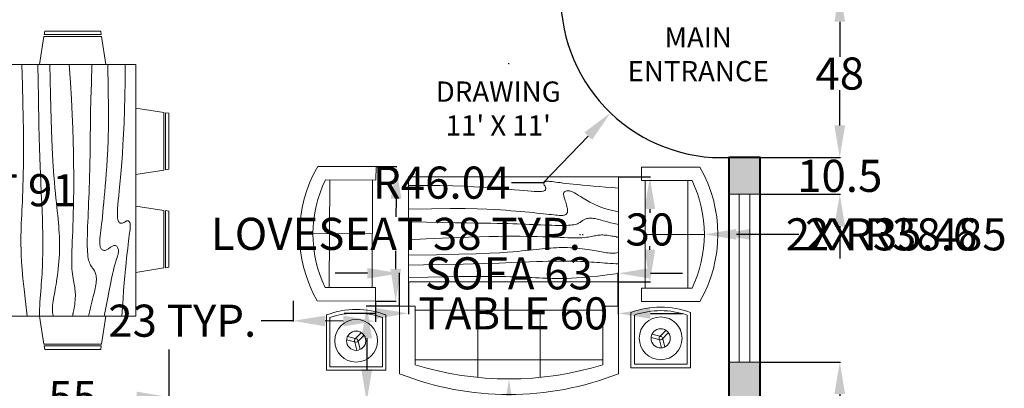
# Model space of a CAD drawing. Units: inches. Extents: x -51 to 563, y -59 to 453.
# Tile 5 of 6: x 211 to 492, y 134 to 240. Entities that reach past the tile are written whole.
import ezdxf

# ---------------------------------------------------------------- set-up
doc = ezdxf.new("R2010")
doc.units = ezdxf.units.IN
doc.header["$MEASUREMENT"] = 0
for name, color, linetype, lineweight in [('A-ANNO-DIMS', 2, 'Continuous', 18), ('A-AREA-IDEN', 7, 'Continuous', 25), ('A-DOOR', 3, 'Continuous', 25), ('A-FURN', 8, 'Continuous', 18), ('A-GLAZ', 4, 'Continuous', 18), ('A-WALL', 7, 'Continuous', 40), ('A-WALL-PATT', 252, 'Continuous', 13)]:
    doc.layers.add(name, color=color, linetype=linetype, lineweight=lineweight)
doc.styles.get("Standard").update_dxf_attribs({"font": 'arial.ttf'})
doc.dimstyles.get("Standard").update_dxf_attribs({"dimtxt": 9.18, "dimasz": 9.18, "dimexe": 0.18, "dimexo": 0.0625, "dimgap": 0.09, "dimtad": 0, "dimtih": 1, "dimtoh": 1, "dimdec": 1, "dimzin": 0, "dimdsep": 46, "dimlunit": 3, "dimtxsty": 'Standard', "dimcen": 0.09, "dimadec": 0, "dimazin": 0, "dimtfac": 1, "dimtdec": 1, "dimtofl": 0, "dimtmove": 0, "dimatfit": 3, "dimfxl": 1, "dimtolj": 1, "dimtzin": 0, "dimarcsym": 0})

# ---------------------------------------------------------------- blocks, each defined once
blk = doc.blocks.new('Dining Set - 36 x 72 in.')
for p, q in [((-22.2343, 26.00059), (-23.4847, 17.99762)), ((-22.2304, 26), (-5.7608, 26)), ((-22, 27.5), (-22.1562, 26.50042)), ((-5.8416, 26.5), (-22.1534, 26.5)), ((-22, 27.5), (-6, 27.5)), ((-5.8437, 26.49966), (-6, 27.5)), ((-4.5152, 17.99762), (-5.7655, 25.99926)), ((5.7657, 26.00059), (4.5153, 17.99762)), ((5.7696, 26), (22.2392, 26)), ((6, 27.5), (5.8438, 26.50042)), ((22.1584, 26.5), (5.8466, 26.5)), ((6, 27.5), (22, 27.5)), ((22.1563, 26.49966), (22, 27.5)), ((23.4848, 17.99762), (22.2345, 25.99926)), ((36, 18), (-36, 18)), ((-36, 18), (-36, -18)), ((36, -18), (36, 18)), ((-44.0006, 8.23428), (-35.9976, 9.48474)), ((44.0006, 8.23428), (35.9976, 9.48474)), ((-45.5, 8), (-44.5004, 8.15617)), ((-45.5, 8), (-45.5, -8)), ((-44.5, -8.15843), (-44.5, 8.15338)), ((-44, 8.23041), (-44, -8.23915)), ((44, 8.23041), (44, -8.23915)), ((44.5, -8.15843), (44.5, 8.15338)), ((45.5, 8), (44.5005, 8.15617)), ((45.5, 8), (45.5, -8)), ((-44.4997, -8.15631), (-45.5, -8)), ((-35.9976, -9.48476), (-43.9993, -8.2345)), ((35.9976, -9.48476), (43.9993, -8.2345)), ((44.4997, -8.15631), (45.5, -8)), ((-36, -18), (36, -18)), ((-22.2343, -26.0006), (-23.4847, -17.99762)), ((-4.5152, -17.99762), (-5.7655, -25.99928)), ((5.7657, -26.0006), (4.5153, -17.99762)), ((23.4848, -17.99762), (22.2345, -25.99928)), ((-22.2304, -26), (-5.7608, -26)), ((-22, -27.5), (-22.1562, -26.50044)), ((-5.8416, -26.5), (-22.1534, -26.5)), ((-22, -27.5), (-6, -27.5)), ((-5.8437, -26.49967), (-6, -27.5)), ((5.7696, -26), (22.2392, -26)), ((6, -27.5), (5.8438, -26.50044)), ((22.1584, -26.5), (5.8466, -26.5)), ((6, -27.5), (22, -27.5)), ((22.1563, -26.49967), (22, -27.5))]:
    blk.add_line(p, q)
for points in [[(-36, 15), (-31.1772, 14.97754), (-26.8079, 14.91406), (-22.8538, 14.81543), (-19.276, 14.6875), (-16.0362, 14.53613), (-13.0957, 14.36718), (-10.4159, 14.18652), (-7.9583, 14), (-5.6904, 13.81315), (-3.6035, 13.63021), (-1.6954, 13.45508), (0.0365, 13.29166), (1.5945, 13.14388), (2.9811, 13.01562), (4.1988, 12.9108), (5.25, 12.83333), (6.1393, 12.78613), (6.8802, 12.76823), (7.4883, 12.77767), (7.9792, 12.8125), (8.3685, 12.87077), (8.6719, 12.95052), (8.9049, 13.0498), (9.0833, 13.16666), (9.2205, 13.29899), (9.3216, 13.44401), (9.3895, 13.59879), (9.4271, 13.76041), (9.4373, 13.92594), (9.4232, 14.09245), (9.3875, 14.257), (9.3333, 14.41666), (9.2638, 14.56917), (9.1836, 14.71484), (9.0975, 14.85465), (9.0104, 14.98958), (8.9272, 15.1206), (8.8529, 15.2487), (8.7922, 15.37483), (8.75, 15.5), (8.7305, 15.62467), (8.7344, 15.74739), (8.7617, 15.86621), (8.8125, 15.97916), (8.8867, 16.08431), (8.9844, 16.17968), (9.1055, 16.26334), (9.25, 16.33333), (9.4189, 16.38802), (9.6172, 16.42708), (9.8506, 16.45052), (10.125, 16.45833), (10.4463, 16.45052), (10.8203, 16.42708), (11.2529, 16.38802), (11.75, 16.33333), (12.3184, 16.26318), (12.9694, 16.17838), (13.7151, 16.07991), (14.5677, 15.96875), (15.5395, 15.84586), (16.6426, 15.71224), (17.8893, 15.56884), (19.2917, 15.41666), (20.859, 15.25667), (22.5879, 15.08984), (24.4721, 14.91715), (26.5052, 14.73958), (28.6809, 14.5581), (30.9929, 14.3737), (33.4347, 14.18733), (36, 14)], [(-36, 10), (-28.9766, 10.14274), (-23.1725, 10.20442), (-18.4241, 10.19775), (-14.5677, 10.13541), (-11.4399, 10.03011), (-8.877, 9.89453), (-6.7154, 9.74137), (-4.7917, 9.58333), (-2.9698, 9.43082), (-1.2246, 9.28515), (0.4415, 9.14534), (2.026, 9.01041), (3.5266, 8.87939), (4.9408, 8.7513), (6.266, 8.62516), (7.5, 8.5), (8.6411, 8.37549), (9.6914, 8.2539), (10.6538, 8.13818), (11.5312, 8.03125), (12.3267, 7.93603), (13.043, 7.85547), (13.6831, 7.79248), (14.25, 7.75), (14.7471, 7.7303), (15.1797, 7.73307), (15.5537, 7.75732), (15.875, 7.80208), (16.1494, 7.86637), (16.3828, 7.94922), (16.5811, 8.04964), (16.75, 8.16666), (16.8944, 8.29915), (17.0143, 8.44531), (17.1089, 8.60319), (17.1771, 8.77083), (17.218, 8.94629), (17.2305, 9.1276), (17.2137, 9.31282), (17.1667, 9.5), (17.0895, 9.6875), (16.987, 9.875), (16.8649, 10.0625), (16.7292, 10.25), (16.5856, 10.4375), (16.4401, 10.625), (16.2985, 10.8125), (16.1667, 11), (16.05, 11.18733), (15.9518, 11.3737), (15.8752, 11.5581), (15.8229, 11.73958), (15.798, 11.91715), (15.8034, 12.08984), (15.842, 12.25667), (15.9167, 12.41666), (16.0295, 12.56836), (16.1784, 12.70833), (16.3605, 12.83268), (16.5729, 12.9375), (16.8127, 13.01888), (17.0768, 13.07291), (17.3625, 13.0957), (17.6667, 13.08333), (17.9894, 13.03312), (18.3418, 12.94726), (18.7382, 12.82918), (19.1927, 12.68229), (19.7195, 12.51001), (20.3327, 12.31575), (21.0465, 12.10294), (21.875, 11.875), (22.8357, 11.63354), (23.959, 11.37304), (25.2786, 11.08618), (26.8282, 10.76562), (28.6414, 10.40405), (30.752, 9.99414), (33.1936, 9.52856), (36, 9)], [(-36, 5.5), (-30.7157, 5.3348), (-26.069, 5.20963), (-21.9946, 5.11767), (-18.4271, 5.05208), (-15.3009, 5.00602), (-12.5508, 4.97265), (-10.1112, 4.94515), (-7.9167, 4.91666), (-5.909, 4.88167), (-4.0586, 4.83984), (-2.3429, 4.79215), (-0.7396, 4.73958), (0.7739, 4.6831), (2.22, 4.6237), (3.6213, 4.56233), (5, 4.5), (6.373, 4.43782), (7.7344, 4.3776), (9.0723, 4.32129), (10.375, 4.27083), (11.6309, 4.22819), (12.8281, 4.19531), (13.9551, 4.17415), (15, 4.16666), (15.954, 4.17448), (16.819, 4.19791), (17.6001, 4.23698), (18.3021, 4.29166), (18.9299, 4.36198), (19.4883, 4.44791), (19.9823, 4.54948), (20.4167, 4.66666), (20.7969, 4.79899), (21.1302, 4.94401), (21.4245, 5.09879), (21.6875, 5.26041), (21.9271, 5.42594), (22.1511, 5.59245), (22.3672, 5.757), (22.5834, 5.91666), (22.8065, 6.06868), (23.0404, 6.21093), (23.2879, 6.34147), (23.5521, 6.45833), (23.8358, 6.55957), (24.142, 6.64323), (24.4735, 6.70735), (24.8334, 6.75), (25.2235, 6.76969), (25.642, 6.76692), (26.0858, 6.74267), (26.5521, 6.69791), (27.0379, 6.63362), (27.5404, 6.55078), (28.0565, 6.45036), (28.5834, 6.33333), (29.1242, 6.19987), (29.7071, 6.04687), (30.3661, 5.87044), (31.1354, 5.66666), (32.0493, 5.43164), (33.142, 5.16146), (34.4475, 4.85221), (36, 4.5)], [(-36, -1), (-30.7915, -0.6591), (-26.0195, -0.38216), (-21.6519, -0.16284), (-17.6563, 0.00521), (-14.0005, 0.12833), (-10.6523, 0.21289), (-7.5796, 0.26522), (-4.75, 0.29166), (-2.134, 0.29793), (0.2878, 0.28711), (2.5317, 0.26163), (4.6146, 0.22396), (6.5529, 0.17651), (8.3633, 0.12174), (10.0623, 0.06209), (11.6667, 0), (13.1899, -0.06201), (14.6341, -0.1211), (15.9982, -0.17432), (17.2813, -0.21875), (18.4823, -0.25147), (19.6003, -0.26953), (20.6343, -0.27002), (21.5834, -0.25), (22.4481, -0.20768), (23.2357, -0.14584), (23.9549, -0.06836), (24.6146, 0.02083), (25.2235, 0.11784), (25.7904, 0.21875), (26.3241, 0.31966), (26.8334, 0.41666), (27.3265, 0.50618), (27.8099, 0.58593), (28.2894, 0.65397), (28.7709, 0.70833), (29.2601, 0.74707), (29.763, 0.76823), (30.2855, 0.76985), (30.8334, 0.75), (31.4088, 0.70784), (31.9994, 0.64713), (32.589, 0.57275), (33.1615, 0.48958), (33.7008, 0.4025), (34.1908, 0.3164), (34.6153, 0.23616), (34.9584, 0.16666), (35.2099, 0.11165), (35.3848, 0.07031), (35.504, 0.04069), (35.5886, 0.02083), (35.6594, 0.00879), (35.7377, 0.0026), (35.8442, 0.00032), (36, 0)], [(-36, -6.5), (-27.1843, -6.31267), (-20.084, -6.1263), (-14.469, -5.9419), (-10.1094, -5.76042), (-6.7752, -5.58285), (-4.2363, -5.41016), (-2.2629, -5.24333), (-0.625, -5.08334), (0.8708, -4.93099), (2.2715, -4.78646), (3.5872, -4.64974), (4.8281, -4.52084), (6.0046, -4.39974), (7.127, -4.28646), (8.2053, -4.18099), (9.25, -4.08334), (10.2705, -3.99382), (11.2734, -3.91407), (12.2647, -3.84603), (13.25, -3.79167), (14.2354, -3.75293), (15.2266, -3.73177), (16.2295, -3.73015), (17.25, -3.75), (18.2912, -3.79248), (19.3451, -3.85547), (20.4009, -3.93604), (21.4479, -4.03125), (22.4754, -4.13819), (23.4727, -4.25391), (24.4289, -4.37549), (25.3334, -4.5), (26.1785, -4.62492), (26.9694, -4.74935), (27.7145, -4.87281), (28.4219, -4.99479), (29.1, -5.11483), (29.7572, -5.23242), (30.4016, -5.34709), (31.0417, -5.45834), (31.6837, -5.56437), (32.3262, -5.65821), (32.9658, -5.73153), (33.599, -5.77604), (34.2224, -5.78345), (34.8327, -5.74545), (35.4264, -5.65373), (36, -5.5)], [(-36, -10), (-26.4022, -9.81299), (-18.4675, -9.62891), (-11.9839, -9.45069), (-6.7396, -9.28125), (-2.5226, -9.12354), (0.8789, -8.98047), (3.6769, -8.85498), (6.0833, -8.75), (8.2767, -8.66765), (10.3021, -8.60677), (12.1712, -8.56543), (13.8958, -8.54167), (15.4876, -8.53353), (16.9583, -8.53907), (18.3197, -8.55632), (19.5834, -8.58334), (20.7616, -8.61841), (21.8685, -8.66081), (22.9188, -8.71004), (23.9271, -8.76563), (24.9081, -8.82707), (25.8763, -8.89388), (26.8465, -8.96558), (27.8334, -9.04167), (28.8474, -9.12118), (29.8828, -9.20117), (30.93, -9.27824), (31.9792, -9.34896), (33.0205, -9.40991), (34.0443, -9.45768), (35.0407, -9.48885), (36, -9.5)], [(-36, -14.5), (-30.0881, -14.33513), (-25.0332, -14.21224), (-20.7312, -14.12647), (-17.0781, -14.07292), (-13.97, -14.04671), (-11.3027, -14.04297), (-8.9724, -14.05681), (-6.875, -14.08334), (-4.9224, -14.11833), (-3.0905, -14.16016), (-1.3709, -14.20785), (0.2448, -14.26042), (1.7647, -14.3169), (3.1973, -14.3763), (4.5507, -14.43767), (5.8333, -14.5), (7.0554, -14.5621), (8.235, -14.62175), (9.3922, -14.67652), (10.5469, -14.72396), (11.7192, -14.76164), (12.929, -14.78711), (14.1965, -14.79794), (15.5417, -14.79167), (16.9933, -14.76424), (18.6152, -14.70508), (20.4804, -14.60197), (22.6615, -14.44271), (25.2312, -14.21509), (28.2624, -13.9069), (31.8277, -13.50594), (36, -13)]]:
    blk.add_lwpolyline(points)
blk = doc.blocks.new('Sofa - Roundback 7 ft.')
for p, q in [((-12.00002, -32.4421), (-12.00003, -6.5971)), ((11.99997, -32.4421), (11.99998, -6.5971)), ((-36.000027, -34), (-36.000027, -11.4696)), ((-35.999844, -13.3819), (35.9998, -13.3819)), ((35.99998, -34), (35.99998, -11.4696)), ((-36.000027, -32.4421), (35.99998, -32.4421))]:
    blk.add_line(p, q)
for points in [[(-36.000027, -34), (-42.000027, -34), (-42.000027, -8)], [(41.99998, -8), (41.99998, -34), (35.99998, -34)]]:
    blk.add_lwpolyline(points)
for centre, radius, start, end in [((0, -114.25), 114.25, 68.43141, 111.5686), ((-0.00001, -127.1968), 121.1968, 72.72033, 107.2797)]:
    blk.add_arc(centre, radius, start, end)
blk = doc.blocks.new('Sofa - Roundback Loveseat 5 ft.')
for p, q in [((0, -32.44198), (0, -5.99998)), ((-24, -33.99998), (-24, -11.46958)), ((24.00004, -33.99998), (24.00004, -11.46958)), ((-23.9998, -13.38178), (23.99986, -13.38178)), ((-24, -32.44198), (24.00004, -32.44198))]:
    blk.add_line(p, q)
for points in [[(-24, -33.99998), (-30, -33.99998), (-30, -7.99998)], [(30.00004, -7.99998), (30.00004, -33.99998), (24.00004, -33.99998)]]:
    blk.add_lwpolyline(points)
for centre, radius, start, end in [((0, -60.24998), 60.24998, 60.13715, 119.8628), ((0, -61.38438), 55.38444, 64.32083, 115.6792)]:
    blk.add_arc(centre, radius, start, end)
blk = doc.blocks.new('Table - Rectangular Woodgrain 60 x 30 in.')
for p, q in [((0, 0), (0, -30)), ((60, 0), (0, 0)), ((60, -30), (60, 0)), ((0, -30), (60, -30))]:
    blk.add_line(p, q)
for points in [[(0, -2.4), (4.8155, -2.418), (9.0302, -2.4688), (12.709, -2.5477), (15.9167, -2.65), (18.7181, -2.7711), (21.1781, -2.9063), (23.3616, -3.0508), (25.3333, -3.2), (27.1477, -3.3495), (28.8172, -3.4958), (30.3437, -3.636), (31.7291, -3.7667), (32.9756, -3.8849), (34.0849, -3.9875), (35.059, -4.0714), (35.9, -4.1334), (36.6114, -4.1711), (37.2041, -4.1854), (37.6906, -4.1779), (38.0833, -4.15), (38.3948, -4.1034), (38.6375, -4.0396), (38.8239, -3.9602), (38.9666, -3.8667), (39.0764, -3.7608), (39.1573, -3.6448), (39.2116, -3.521), (39.2416, -3.3917), (39.2498, -3.2593), (39.2385, -3.1261), (39.21, -2.9944), (39.1666, -2.8667), (39.111, -2.7447), (39.0468, -2.6281), (38.978, -2.5163), (38.9083, -2.4083), (38.8418, -2.3035), (38.7823, -2.201), (38.7337, -2.1001), (38.7, -2), (38.6844, -1.9003), (38.6875, -1.8021), (38.7094, -1.707), (38.75, -1.6167), (38.8094, -1.5326), (38.8875, -1.4563), (38.9844, -1.3893), (39.1, -1.3333), (39.2351, -1.2896), (39.3937, -1.2583), (39.5804, -1.2396), (39.8, -1.2333), (40.057, -1.2396), (40.3562, -1.2583), (40.7023, -1.2896), (41.1, -1.3333), (41.5547, -1.3895), (42.0755, -1.4573), (42.6721, -1.5361), (43.3542, -1.625), (44.1316, -1.7233), (45.014, -1.8302), (46.0114, -1.9449), (47.1333, -2.0667), (48.3862, -2.1947), (49.7625, -2.3281), (51.2513, -2.4663), (52.8416, -2.6083), (54.5226, -2.7535), (56.2833, -2.9011), (58.1127, -3.0501), (60, -3.2)], [(0, -9.2), (6.5759, -9.0858), (11.9385, -9.0365), (16.2527, -9.0418), (19.6833, -9.0917), (22.3952, -9.1759), (24.5531, -9.2844), (26.322, -9.4069), (27.8666, -9.5333), (29.3241, -9.6553), (30.7203, -9.7719), (32.0532, -9.8837), (33.3208, -9.9917), (34.5213, -10.0965), (35.6526, -10.199), (36.7128, -10.2999), (37.7, -10.4), (38.6129, -10.4996), (39.4531, -10.5969), (40.223, -10.6895), (40.925, -10.775), (41.5613, -10.8512), (42.1344, -10.9156), (42.6465, -10.966), (43.1, -11), (43.4976, -11.0158), (43.8437, -11.0136), (44.143, -10.9942), (44.4, -10.9583), (44.6195, -10.9069), (44.8062, -10.8406), (44.9648, -10.7603), (45.1, -10.6667), (45.2155, -10.5598), (45.3114, -10.4365), (45.3871, -10.2929), (45.4416, -10.125), (45.4743, -9.929), (45.4844, -9.7011), (45.4709, -9.4371), (45.4333, -9.1333), (45.3716, -8.7883), (45.2896, -8.4104), (45.1919, -8.0107), (45.0833, -7.6), (44.9685, -7.1893), (44.8521, -6.7896), (44.7388, -6.4117), (44.6333, -6.0667), (44.54, -5.7628), (44.4614, -5.4979), (44.4001, -5.2675), (44.3583, -5.0667), (44.3384, -4.8909), (44.3427, -4.7354), (44.3736, -4.5956), (44.4333, -4.4667), (44.5236, -4.3453), (44.6427, -4.2333), (44.7884, -4.1339), (44.9583, -4.05), (45.1501, -3.9849), (45.3614, -3.9417), (45.59, -3.9234), (45.8333, -3.9333), (46.0915, -3.9749), (46.3734, -4.0531), (46.6906, -4.1736), (47.0542, -4.3417), (47.4756, -4.5629), (47.9661, -4.8427), (48.5372, -5.1866), (49.2, -5.6), (49.9676, -6.0844), (50.8594, -6.625), (51.8965, -7.2031), (53.1, -7.8), (54.491, -8.3969), (56.0906, -8.975), (57.9199, -9.5156), (60, -10)], [(0, -12.8), (5.1847, -12.9322), (9.6213, -13.0323), (13.3963, -13.1059), (16.5958, -13.1583), (19.3063, -13.1952), (21.614, -13.2219), (23.6054, -13.2439), (25.3666, -13.2667), (26.9728, -13.2947), (28.4531, -13.3281), (29.8256, -13.3663), (31.1083, -13.4083), (32.3191, -13.4535), (33.476, -13.501), (34.597, -13.5501), (35.7, -13.6), (36.7984, -13.6497), (37.8875, -13.6979), (38.9578, -13.743), (40, -13.7833), (41.0047, -13.8174), (41.9625, -13.8438), (42.864, -13.8607), (43.7, -13.8667), (44.4631, -13.8604), (45.1552, -13.8417), (45.7801, -13.8104), (46.3416, -13.7667), (46.8439, -13.7104), (47.2906, -13.6417), (47.6858, -13.5604), (48.0333, -13.4667), (48.3375, -13.3608), (48.6042, -13.2448), (48.8396, -13.121), (49.05, -12.9917), (49.2417, -12.8593), (49.4208, -12.7261), (49.5937, -12.5944), (49.7667, -12.4667), (49.9452, -12.3451), (50.1323, -12.2313), (50.3303, -12.1268), (50.5416, -12.0333), (50.7686, -11.9524), (51.0135, -11.8854), (51.2788, -11.8341), (51.5666, -11.8), (51.8785, -11.7843), (52.2116, -11.7865), (52.562, -11.8059), (52.926, -11.8417), (53.2998, -11.8931), (53.6795, -11.9594), (54.0614, -12.0397), (54.4416, -12.1333), (54.8223, -12.2401), (55.2293, -12.3625), (55.6942, -12.5037), (56.2489, -12.6667), (56.9251, -12.8547), (57.7545, -13.0708), (58.7689, -13.3182), (60, -13.6)], [(0, -18), (5.124, -17.7273), (9.6609, -17.5057), (13.6705, -17.3303), (17.2125, -17.1958), (20.3467, -17.0973), (23.1328, -17.0297), (25.6307, -16.9878), (27.9, -16.9667), (29.9928, -16.9617), (31.9302, -16.9703), (33.7254, -16.9907), (35.3917, -17.0208), (36.9423, -17.0588), (38.3906, -17.1026), (39.7499, -17.1503), (41.0333, -17.2), (42.2519, -17.2496), (43.4073, -17.2969), (44.4986, -17.3395), (45.525, -17.375), (46.4858, -17.4012), (47.3802, -17.4156), (48.2074, -17.416), (48.9667, -17.4), (49.6583, -17.3662), (50.2872, -17.3167), (50.8595, -17.2547), (51.3812, -17.1833), (51.8584, -17.1057), (52.2971, -17.025), (52.7034, -16.9443), (53.0833, -16.8667), (53.443, -16.7951), (53.789, -16.7313), (54.128, -16.6768), (54.4666, -16.6334), (54.8115, -16.6024), (55.1693, -16.5854), (55.5465, -16.5841), (55.95, -16.6), (56.3828, -16.6337), (56.8346, -16.6823), (57.2915, -16.7418), (57.7396, -16.8084), (58.165, -16.878), (58.5539, -16.9469), (58.8924, -17.0111), (59.1666, -17.0667), (59.3679, -17.1107), (59.5078, -17.1438), (59.6032, -17.1675), (59.6708, -17.1833), (59.7275, -17.193), (59.7901, -17.1979), (59.8753, -17.1998), (60, -17.2)], [(0, -22.4), (8.0098, -22.2501), (14.4094, -22.1011), (19.4168, -21.9535), (23.25, -21.8083), (26.1269, -21.6663), (28.2656, -21.5281), (29.884, -21.3947), (31.2, -21.2667), (32.3967, -21.1448), (33.5172, -21.0292), (34.5697, -20.9198), (35.5625, -20.8167), (36.5037, -20.7198), (37.4015, -20.6292), (38.2642, -20.5448), (39.1, -20.4667), (39.9164, -20.3951), (40.7187, -20.3313), (41.5117, -20.2768), (42.3, -20.2333), (43.0883, -20.2024), (43.8812, -20.1854), (44.6836, -20.1841), (45.5, -20.2), (46.3328, -20.234), (47.1747, -20.2844), (48.0163, -20.3488), (48.8479, -20.425), (49.66, -20.5106), (50.4429, -20.6031), (51.1872, -20.7004), (51.8833, -20.8), (52.5246, -20.8999), (53.1166, -20.9995), (53.6681, -21.0983), (54.1875, -21.1958), (54.6834, -21.2919), (55.1646, -21.3859), (55.6394, -21.4777), (56.1167, -21.5667), (56.6028, -21.6515), (57.0961, -21.7266), (57.5929, -21.7852), (58.0896, -21.8208), (58.5823, -21.8268), (59.0674, -21.7964), (59.5412, -21.723), (60, -21.6)], [(0, -25.2), (8.6355, -25.0504), (15.7026, -24.9031), (21.4049, -24.7606), (25.9458, -24.625), (29.529, -24.4988), (32.3578, -24.3844), (34.6359, -24.284), (36.5667, -24.2), (38.3213, -24.1341), (39.9417, -24.0854), (41.437, -24.0523), (42.8167, -24.0333), (44.0901, -24.0268), (45.2667, -24.0313), (46.3557, -24.0451), (47.3667, -24.0667), (48.309, -24.0947), (49.1928, -24.1287), (50.0284, -24.168), (50.826, -24.2125), (51.5959, -24.2617), (52.3483, -24.3151), (53.0935, -24.3725), (53.8417, -24.4334), (54.6009, -24.497), (55.3699, -24.561), (56.1454, -24.6226), (56.9239, -24.6792), (57.7021, -24.7279), (58.4764, -24.7662), (59.2435, -24.7911), (60, -24.8)], [(0, -28.8), (5.6867, -28.6681), (10.45, -28.5698), (14.407, -28.5012), (17.675, -28.4584), (20.3711, -28.4374), (22.6125, -28.4344), (24.5164, -28.4455), (26.2, -28.4667), (27.762, -28.4947), (29.2276, -28.5281), (30.6033, -28.5663), (31.8958, -28.6084), (33.1118, -28.6535), (34.2578, -28.7011), (35.3405, -28.7501), (36.3666, -28.8), (37.3443, -28.8497), (38.288, -28.8974), (39.2137, -28.9412), (40.1375, -28.9792), (41.0753, -29.0093), (42.0432, -29.0297), (43.0572, -29.0384), (44.1333, -29.0333), (45.2936, -29.0114), (46.5843, -28.9641), (48.0579, -28.8816), (49.7666, -28.7542), (51.7629, -28.5721), (54.0989, -28.3255), (56.8272, -28.0048), (60, -27.6)]]:
    blk.add_lwpolyline(points)
blk = doc.blocks.new('WIN-48IN')
for p, q in [((9, 48), (0, 48)), ((3, 48), (3, 0)), ((6, 48), (6, 0)), ((9, 0), (0, 0))]:
    blk.add_line(p, q)
blk = doc.blocks.new('*U11')
for p, q in [((-1.31, -0.61), (0.61, 1.31)), ((-0.61, -1.31), (1.31, 0.61))]:
    blk.add_line(p, q)
blk = doc.blocks.new('*U12')
at = {"color": 0, "linetype": 'ByBlock', "lineweight": -2, "transparency": 16777216}
for p, rotation in [((276.07, -10.08), 120), ((277.73, -11.74), 239.9999999999999)]:
    blk.add_blockref('*U11', p, dxfattribs=dict(at, rotation=rotation))
blk.add_blockref('*U11', (278.34, -9.47), dxfattribs=at)
blk = doc.blocks.new('TABLE-SIDE-WITH-LAMP')
for points in [[(17.03, 15.79), (17.03, 0), (0, 0), (0, 15.79, -0.18199)], [(16.03, 15.08), (16.03, 1), (1, 1), (1, 15.08, -0.16668)]]:
    blk.add_lwpolyline(points, format="xyb", close=True)
for centre, radius in [((8.51, 8.42), 6.11), ((8.51, 8.42), 2.75), ((8.51, 8.47), 0.5)]:
    blk.add_circle(centre, radius)
blk.add_blockref('*U12', (-268.87, 18.9))
blk = doc.blocks.new('*D29')
at = {"layer": 'A-ANNO-DIMS', "color": 0, "lineweight": -2, "transparency": 16777216}
for p, q in [((312.82, 197.75), (318.7, 197.73)), ((318.48, 188.55), (318.46, 183.35)), ((318.4, 168.46), (318.42, 173.66)), ((312.66, 159.31), (318.54, 159.28))]:
    blk.add_line(p, q, dxfattribs=at)
at = {"layer": 'A-ANNO-DIMS', "color": 0, "transparency": 16777216}
for points in [[(316.95, 188.55), (320.01, 188.54), (318.52, 197.73)], [(316.87, 168.47), (319.93, 168.46), (318.36, 159.28)]]:
    blk.add_solid(points, dxfattribs=at)
at = {"layer": 'Defpoints', "color": 0, "transparency": 16777216}
for p in [(312.76, 197.75), (312.6, 159.31), (318.36, 159.28)]:
    blk.add_point(p, dxfattribs=at)
at = {"layer": 'A-ANNO-DIMS', "color": 0, "transparency": 16777216, "insert": (318.44, 178.51), "char_height": 9.18, "attachment_point": 5}
blk.add_mtext('\\A1;LOVESEAT 38 TYP.', dxfattribs=at)
blk = doc.blocks.new('*D30')
at = {"layer": 'A-ANNO-DIMS', "color": 0, "lineweight": -2, "transparency": 16777216}
for p, q in [((289.11, 159.34), (289.08, 153.46)), ((312.6, 159.25), (312.57, 153.36)), ((289.08, 153.64), (279.9, 153.68)), ((303.39, 153.58), (298.26, 153.6))]:
    blk.add_line(p, q, dxfattribs=at)
at = {"layer": 'A-ANNO-DIMS', "color": 0, "transparency": 16777216}
for points in [[(298.27, 155.13), (298.26, 152.07), (289.08, 153.64)], [(303.4, 155.11), (303.39, 152.05), (312.57, 153.54)]]:
    blk.add_solid(points, dxfattribs=at)
at = {"layer": 'Defpoints', "color": 0, "transparency": 16777216}
for p in [(289.11, 159.41), (312.6, 159.31), (289.08, 153.64)]:
    blk.add_point(p, dxfattribs=at)
at = {"layer": 'A-ANNO-DIMS', "color": 0, "transparency": 16777216, "insert": (257.39, 153.68), "char_height": 9.18, "attachment_point": 5}
blk.add_mtext('\\A1;23 TYP.', dxfattribs=at)
blk = doc.blocks.new('*D35')
at = {"layer": 'A-ANNO-DIMS', "color": 0, "lineweight": -2, "transparency": 16777216}
for p, q in [((310.3, 167.23), (301.12, 167.23)), ((319.48, 157.91), (319.48, 167.41)), ((381.99, 157.91), (381.99, 167.41)), ((391.17, 167.23), (400.35, 167.23))]:
    blk.add_line(p, q, dxfattribs=at)
at = {"layer": 'A-ANNO-DIMS', "color": 0, "transparency": 16777216}
for points in [[(310.3, 168.76), (310.3, 165.7), (319.48, 167.23)], [(391.17, 168.76), (391.17, 165.7), (381.99, 167.23)]]:
    blk.add_solid(points, dxfattribs=at)
at = {"layer": 'Defpoints', "color": 0, "transparency": 16777216}
for p in [(319.48, 167.23), (319.48, 157.85), (381.99, 157.85)]:
    blk.add_point(p, dxfattribs=at)
at = {"layer": 'A-ANNO-DIMS', "color": 0, "transparency": 16777216, "insert": (350.74, 167.23), "char_height": 9.18, "attachment_point": 5}
blk.add_mtext('\\A1;SOFA 63', dxfattribs=at)
blk = doc.blocks.new('*D36')
at = {"layer": 'A-ANNO-DIMS', "color": 0, "lineweight": -2, "transparency": 16777216}
for p, q in [((319.42, 157.85), (309.92, 157.85)), ((310.1, 148.67), (310.1, 139.74)), ((319.42, 130.56), (309.92, 130.56)), ((310.1, 130.56), (310.1, 121.38)), ((310.1, 121.38), (300.92, 121.38))]:
    blk.add_line(p, q, dxfattribs=at)
at = {"layer": 'A-ANNO-DIMS', "color": 0, "transparency": 16777216}
for points in [[(308.57, 148.67), (311.63, 148.67), (310.1, 157.85)], [(308.57, 139.74), (311.63, 139.74), (310.1, 130.56)]]:
    blk.add_solid(points, dxfattribs=at)
at = {"layer": 'Defpoints', "color": 0, "transparency": 16777216}
for p in [(319.48, 157.85), (310.1, 130.56), (319.48, 130.56)]:
    blk.add_point(p, dxfattribs=at)
at = {"layer": 'A-ANNO-DIMS', "color": 0, "transparency": 16777216, "insert": (294.18, 121.38), "char_height": 9.18, "attachment_point": 5}
blk.add_mtext('\\A1;27', dxfattribs=at)
blk = doc.blocks.new('*D49')
at = {"layer": 'A-ANNO-DIMS', "color": 0, "lineweight": -2, "transparency": 16777216}
for p, q in [((246.41, 117), (246.41, 126.18)), ((246.41, 126.18), (255.59, 126.18)), ((243.43, 117), (246.59, 117)), ((246.41, 105.95), (246.41, 107.82)), ((243.43, 96.77), (246.59, 96.77))]:
    blk.add_line(p, q, dxfattribs=at)
at = {"layer": 'A-ANNO-DIMS', "color": 0, "transparency": 16777216}
for points in [[(244.88, 107.82), (247.94, 107.82), (246.41, 117)], [(244.88, 105.95), (247.94, 105.95), (246.41, 96.77)]]:
    blk.add_solid(points, dxfattribs=at)
at = {"layer": 'Defpoints', "color": 0, "transparency": 16777216}
for p in [(243.37, 117), (246.41, 117), (243.37, 96.77)]:
    blk.add_point(p, dxfattribs=at)
at = {"layer": 'A-ANNO-DIMS', "color": 0, "transparency": 16777216, "insert": (283.06, 126.18), "char_height": 9.18, "attachment_point": 5}
blk.add_mtext('\\A1;BASIN 20', dxfattribs=at)
blk = doc.blocks.new('*D57')
at = {"layer": 'A-ANNO-DIMS', "color": 0, "lineweight": -2, "transparency": 16777216}
for p, q in [((198.52, 236.49), (184.76, 236.49)), ((184.94, 227.31), (184.94, 195.82)), ((184.94, 154.67), (184.94, 186.15)), ((198.52, 145.49), (184.76, 145.49))]:
    blk.add_line(p, q, dxfattribs=at)
at = {"layer": 'A-ANNO-DIMS', "color": 0, "transparency": 16777216}
for points in [[(183.41, 227.31), (186.47, 227.31), (184.94, 236.49)], [(183.41, 154.67), (186.47, 154.67), (184.94, 145.49)]]:
    blk.add_solid(points, dxfattribs=at)
at = {"layer": 'Defpoints', "color": 0, "transparency": 16777216}
for p in [(198.59, 236.49), (184.94, 145.49), (198.59, 145.49)]:
    blk.add_point(p, dxfattribs=at)
at = {"layer": 'A-ANNO-DIMS', "color": 0, "transparency": 16777216, "insert": (184.94, 190.99), "char_height": 9.18, "attachment_point": 5}
blk.add_mtext('\\A1;DINING SET 91', dxfattribs=at)
blk = doc.blocks.new('*D58')
at = {"layer": 'A-ANNO-DIMS', "color": 0, "lineweight": -2, "transparency": 16777216}
for p, q in [((198.59, 145.43), (198.59, 131.66)), ((253.59, 145.43), (253.59, 131.66)), ((207.77, 131.84), (219.39, 131.84)), ((244.41, 131.84), (232.79, 131.84))]:
    blk.add_line(p, q, dxfattribs=at)
at = {"layer": 'A-ANNO-DIMS', "color": 0, "transparency": 16777216}
for points in [[(207.77, 133.37), (207.77, 130.31), (198.59, 131.84)], [(244.41, 133.37), (244.41, 130.31), (253.59, 131.84)]]:
    blk.add_solid(points, dxfattribs=at)
at = {"layer": 'Defpoints', "color": 0, "transparency": 16777216}
for p in [(198.59, 145.49), (253.59, 145.49), (253.59, 131.84)]:
    blk.add_point(p, dxfattribs=at)
at = {"layer": 'A-ANNO-DIMS', "color": 0, "transparency": 16777216, "insert": (226.09, 131.84), "char_height": 9.18, "attachment_point": 5}
blk.add_mtext('\\A1;55', dxfattribs=at)
blk = doc.blocks.new('*D61')
at = {"layer": 'A-ANNO-DIMS', "color": 0, "lineweight": -2, "transparency": 16777216}
for p, q in [((321.99, 164.71), (321.99, 155.59)), ((381.99, 164.71), (381.99, 155.59)), ((312.81, 155.77), (303.63, 155.77)), ((391.17, 155.77), (400.35, 155.77))]:
    blk.add_line(p, q, dxfattribs=at)
at = {"layer": 'A-ANNO-DIMS', "color": 0, "transparency": 16777216}
for points in [[(312.81, 157.3), (312.81, 154.24), (321.99, 155.77)], [(391.17, 157.3), (391.17, 154.24), (381.99, 155.77)]]:
    blk.add_solid(points, dxfattribs=at)
at = {"layer": 'Defpoints', "color": 0, "transparency": 16777216}
for p in [(321.99, 164.77), (381.99, 164.77), (381.99, 155.77)]:
    blk.add_point(p, dxfattribs=at)
at = {"layer": 'A-ANNO-DIMS', "color": 0, "transparency": 16777216, "insert": (351.99, 155.77), "char_height": 9.18, "attachment_point": 5}
blk.add_mtext('\\A1;TABLE 60', dxfattribs=at)
blk = doc.blocks.new('*D62')
at = {"layer": 'A-ANNO-DIMS', "color": 0, "lineweight": -2, "transparency": 16777216}
for p, q in [((382.06, 194.77), (391.17, 194.77)), ((390.99, 185.59), (390.99, 184.55)), ((390.99, 173.95), (390.99, 174.99)), ((382.06, 164.77), (391.17, 164.77))]:
    blk.add_line(p, q, dxfattribs=at)
at = {"layer": 'A-ANNO-DIMS', "color": 0, "transparency": 16777216}
for points in [[(389.46, 185.59), (392.52, 185.59), (390.99, 194.77)], [(389.46, 173.95), (392.52, 173.95), (390.99, 164.77)]]:
    blk.add_solid(points, dxfattribs=at)
at = {"layer": 'Defpoints', "color": 0, "transparency": 16777216}
for p in [(381.99, 194.77), (390.99, 194.77), (381.99, 164.77)]:
    blk.add_point(p, dxfattribs=at)
at = {"layer": 'A-ANNO-DIMS', "color": 0, "transparency": 16777216, "insert": (390.99, 179.77), "char_height": 9.18, "attachment_point": 5}
blk.add_mtext('\\A1;30', dxfattribs=at)
blk = doc.blocks.new('*D70')
at = {"layer": 'A-ANNO-DIMS', "color": 0, "lineweight": -2, "transparency": 16777216}
for p, q in [((422.62, 248.35), (445.44, 248.35)), ((445.26, 239.17), (445.26, 229.12)), ((445.26, 209.53), (445.26, 219.57)), ((422.62, 200.35), (445.44, 200.35))]:
    blk.add_line(p, q, dxfattribs=at)
at = {"layer": 'A-ANNO-DIMS', "color": 0, "transparency": 16777216}
for points in [[(443.73, 239.17), (446.79, 239.17), (445.26, 248.35)], [(443.73, 209.53), (446.79, 209.53), (445.26, 200.35)]]:
    blk.add_solid(points, dxfattribs=at)
at = {"layer": 'Defpoints', "color": 0, "transparency": 16777216}
for p in [(422.56, 248.35), (422.56, 200.35), (445.26, 200.35)]:
    blk.add_point(p, dxfattribs=at)
at = {"layer": 'A-ANNO-DIMS', "color": 0, "transparency": 16777216, "insert": (445.26, 224.35), "char_height": 9.18, "attachment_point": 5}
blk.add_mtext('\\A1;48', dxfattribs=at)
blk = doc.blocks.new('*D71')
at = {"layer": 'A-ANNO-DIMS', "color": 0, "lineweight": -2, "transparency": 16777216}
for p, q in [((445.258368, 209.527899), (445.258368, 218.707899)), ((422.620868, 200.347899), (445.438368, 200.347899)), ((422.620868, 189.847899), (445.438368, 189.847899)), ((445.258368, 180.667899), (445.258368, 171.487899))]:
    blk.add_line(p, q, dxfattribs=at)
at = {"layer": 'A-ANNO-DIMS', "color": 0, "transparency": 16777216}
for points in [[(443.728368, 209.527899), (446.788368, 209.527899), (445.258368, 200.347899)], [(443.728368, 180.667899), (446.788368, 180.667899), (445.258368, 189.847899)]]:
    blk.add_solid(points, dxfattribs=at)
at = {"layer": 'Defpoints', "color": 0, "transparency": 16777216}
for p in [(422.558368, 200.347899), (422.558368, 189.847899), (445.258368, 189.847899)]:
    blk.add_point(p, dxfattribs=at)
at = {"layer": 'A-ANNO-DIMS', "color": 0, "transparency": 16777216, "insert": (445.258368, 195.097899), "char_height": 9.18, "attachment_point": 5}
blk.add_mtext('\\A1;10.5', dxfattribs=at)
blk = doc.blocks.new('*D72')
at = {"layer": 'A-ANNO-DIMS', "color": 0, "lineweight": -2, "transparency": 16777216}
for p, q in [((422.62, 141.85), (445.44, 141.85)), ((445.26, 132.67), (445.26, 60.37)), ((445.26, -21.47), (445.26, 50.82)), ((422.62, -30.65), (445.44, -30.65))]:
    blk.add_line(p, q, dxfattribs=at)
at = {"layer": 'A-ANNO-DIMS', "color": 0, "transparency": 16777216}
for points in [[(443.73, 132.67), (446.79, 132.67), (445.26, 141.85)], [(443.73, -21.47), (446.79, -21.47), (445.26, -30.65)]]:
    blk.add_solid(points, dxfattribs=at)
at = {"layer": 'Defpoints', "color": 0, "transparency": 16777216}
for p in [(422.56, 141.85), (422.56, -30.65), (445.26, -30.65)]:
    blk.add_point(p, dxfattribs=at)
at = {"layer": 'A-ANNO-DIMS', "color": 0, "transparency": 16777216, "insert": (445.26, 55.6), "char_height": 9.18, "attachment_point": 5}
blk.add_mtext('\\A1;172.5', dxfattribs=at)
blk = doc.blocks.new('*D81')
at = {"layer": 'A-ANNO-DIMS', "color": 0, "lineweight": -2, "transparency": 16777216}
for p, q in [((411.51, 246.35), (411.69, 246.35)), ((411.6, 246.26), (411.6, 246.44)), ((360.63, 193.16), (373.39, 206.48)), ((351.45, 193.16), (360.63, 193.16))]:
    blk.add_line(p, q, dxfattribs=at)
at = {"layer": 'A-ANNO-DIMS', "color": 0, "transparency": 16777216}
blk.add_solid([(372.29, 207.54), (374.5, 205.42), (379.74, 213.11)], dxfattribs=at)
at = {"layer": 'Defpoints', "color": 0, "transparency": 16777216}
for p in [(411.6, 246.35), (379.74, 213.11)]:
    blk.add_point(p, dxfattribs=at)
at = {"layer": 'A-ANNO-DIMS', "color": 0, "transparency": 16777216, "insert": (331.5, 193.16), "char_height": 9.18, "attachment_point": 5}
blk.add_mtext('\\A1;R46.04', dxfattribs=at)
blk = doc.blocks.new('*D91')
at = {"layer": 'A-ANNO-DIMS', "color": 0, "lineweight": -2, "transparency": 16777216}
for p, q in [((350.65, 227.21), (350.83, 227.21)), ((350.74, 227.12), (350.74, 227.3)), ((350.74, 82.9), (350.74, 127.83)), ((359.92, 82.9), (350.74, 82.9))]:
    blk.add_line(p, q, dxfattribs=at)
at = {"layer": 'A-ANNO-DIMS', "color": 0, "transparency": 16777216}
blk.add_solid([(352.27, 127.83), (349.21, 127.83), (350.74, 137.01)], dxfattribs=at)
at = {"layer": 'Defpoints', "color": 0, "transparency": 16777216}
for p in [(350.74, 227.21), (350.74, 137.01)]:
    blk.add_point(p, dxfattribs=at)
at = {"layer": 'A-ANNO-DIMS', "color": 0, "transparency": 16777216, "insert": (376.27, 82.9), "char_height": 9.18, "attachment_point": 5}
blk.add_mtext('\\A1;R90.2', dxfattribs=at)
blk = doc.blocks.new('*D92')
at = {"layer": 'A-ANNO-DIMS', "color": 0, "lineweight": -2, "transparency": 16777216}
for p, q in [((350.65, 217.57), (350.83, 217.57)), ((350.74, 217.48), (350.74, 217.66)), ((350.74, 81.53), (350.74, 123.37)), ((359.92, 81.53), (350.74, 81.53))]:
    blk.add_line(p, q, dxfattribs=at)
at = {"layer": 'A-ANNO-DIMS', "color": 0, "transparency": 16777216}
blk.add_solid([(352.27, 123.37), (349.21, 123.37), (350.74, 132.55)], dxfattribs=at)
at = {"layer": 'Defpoints', "color": 0, "transparency": 16777216}
for p in [(350.74, 217.57), (350.74, 132.55)]:
    blk.add_point(p, dxfattribs=at)
at = {"layer": 'A-ANNO-DIMS', "color": 0, "transparency": 16777216, "insert": (379.84, 81.53), "char_height": 9.18, "attachment_point": 5}
blk.add_mtext('\\A1;R85.02', dxfattribs=at)
blk = doc.blocks.new('*D95')
at = {"layer": 'A-ANNO-DIMS', "color": 0, "lineweight": -2, "transparency": 16777216}
for p, q in [((371.73, 178.37), (371.91, 178.37)), ((371.82, 178.28), (371.82, 178.46)), ((433.58, 178.37), (419.6, 178.37))]:
    blk.add_line(p, q, dxfattribs=at)
at = {"layer": 'A-ANNO-DIMS', "color": 0, "transparency": 16777216}
blk.add_solid([(419.6, 179.9), (419.6, 176.84), (410.42, 178.37)], dxfattribs=at)
at = {"layer": 'Defpoints', "color": 0, "transparency": 16777216}
for p in [(371.82, 178.37), (410.42, 178.37)]:
    blk.add_point(p, dxfattribs=at)
at = {"layer": 'A-ANNO-DIMS', "color": 0, "transparency": 16777216, "insert": (459.92, 178.37), "char_height": 9.18, "attachment_point": 5}
blk.add_mtext('\\A1;2X R38.6', dxfattribs=at)
blk = doc.blocks.new('*D96')
at = {"layer": 'A-ANNO-DIMS', "color": 0, "lineweight": -2, "transparency": 16777216}
for p, q in [((371, 178.37), (371.18, 178.37)), ((371.09, 178.28), (371.09, 178.46)), ((427.86, 178.37), (415.75, 178.37))]:
    blk.add_line(p, q, dxfattribs=at)
at = {"layer": 'A-ANNO-DIMS', "color": 0, "transparency": 16777216}
blk.add_solid([(415.75, 179.9), (415.75, 176.84), (406.57, 178.37)], dxfattribs=at)
at = {"layer": 'Defpoints', "color": 0, "transparency": 16777216}
for p in [(371.09, 178.37), (406.57, 178.37)]:
    blk.add_point(p, dxfattribs=at)
at = {"layer": 'A-ANNO-DIMS', "color": 0, "transparency": 16777216, "insert": (461.38, 178.37), "char_height": 9.18, "attachment_point": 5}
blk.add_mtext('\\A1;2X R35.485', dxfattribs=at)

msp = doc.modelspace()

# ---------------------------------------------------------------- linework, layer by layer
at = {"layer": 'A-DOOR'}
msp.add_arc((411.6, 246.3479), 46.0417, 180, 272.43775, dxfattribs=at)
at = {"layer": 'A-WALL'}
msp.add_lwpolyline([(35.5584, -30.6521), (284.5584, -30.6521), (413.5584, -30.6521), (422.5584, -30.6521), (422.5584, 0.8479), (422.5584, 200.3479), (413.5584, 200.3479), (413.5584, 131.3479), (287.5584, 131.3479), (287.5584, 126.8479), (413.5584, 126.8479), (413.5584, -21.6521), (284.5584, -21.6521), (248.5584, -21.6521), (248.5584, 14.3479), (244.0584, 14.3479), (244.0584, -21.6521), (184.0584, -21.6521)], dxfattribs=at)
at = {"layer": 'A-WALL-PATT'}
for points in [[(413.5584, 189.8479), (422.5584, 189.8479), (413.5584, 200.3479), (422.5584, 200.3479)], [(413.5584, -21.6521), (422.5584, -30.6521), (413.5584, 141.8479), (422.5584, 141.8479)]]:
    msp.add_solid(points, dxfattribs=at)

# ---------------------------------------------------------------- block references
at = {"layer": 'A-FURN', "rotation": 270}
msp.add_blockref('Dining Set - 36 x 72 in.', (226.0874, 190.988), dxfattribs=at)
at = {"layer": 'A-FURN'}
for name, p, xscale, yscale, zscale, rotation in [('Sofa - Roundback Loveseat 5 ft.', (290.8935, 178.6189), -0.6406989062012184, 0.6406989062012184, 0.6406989062012184, 89.76436789404735), ('Sofa - Roundback Loveseat 5 ft.', (410.4171, 178.3731), 0.6406989062012184, 0.6406989062012184, 0.6406989062012184, 270), ('Sofa - Roundback 7 ft.', (350.7357, 132.5493), 0.7442004743752547, 0.7442004743752547, 0.7442004743752547, 180)]:
    msp.add_blockref(name, p, dxfattribs=dict(at, xscale=xscale, yscale=yscale, zscale=zscale, rotation=rotation))
for name, p in [('Table - Rectangular Woodgrain 60 x 30 in.', (321.994, 194.7746)), ('TABLE-SIDE-WITH-LAMP', (385.581, 140.2198)), ('TABLE-SIDE-WITH-LAMP', (298.5727, 139.5289))]:
    msp.add_blockref(name, p, dxfattribs=at)
at = {"layer": 'A-GLAZ', "rotation": 180}
msp.add_blockref('WIN-48IN', (422.5587, 189.8478), dxfattribs=at)

# ---------------------------------------------------------------- texts
at = {"layer": 'A-AREA-IDEN', "char_height": 5.8, "attachment_point": 1}
for s, insert in [('\\pxqc;MAIN\\PENTRANCE', (380.0209, 237.6073)), ("\\pxqc;DRAWING\\P11' X 11'", (322.8826, 222.0828))]:
    msp.add_mtext_dynamic_manual_height_columns(s, width=49.588896, gutter_width=1, heights=[0], dxfattribs=dict(at, insert=insert))

# ---------------------------------------------------------------- dimensions: what is measured, and where the dimension line sits
at = {"layer": 'A-ANNO-DIMS'}
for base, p1, p2, angle, override, picture, middle in [((445.2584, 200.3479), (422.5584, 248.3479), (422.5584, 200.3479), 90, {"dimdec": 0, "dimlfac": 1, "dimrnd": 0, "dimzin": 0, "dimdsep": 46, "dimlunit": 2}, '*D70', (445.2584, 224.3479)), ((445.2584, 189.8479), (422.5584, 200.3479), (422.5584, 189.8479), 90, {"dimdec": 1, "dimlfac": 1, "dimrnd": 0, "dimzin": 0, "dimdsep": 46, "dimlunit": 2}, '*D71', (445.2584, 195.0979)), ((390.994, 194.7746), (381.994, 164.7746), (381.994, 194.7746), 90, {"dimdec": 0, "dimlfac": 1, "dimrnd": 0, "dimzin": 0, "dimdsep": 46, "dimlunit": 2}, '*D62', (390.994, 179.7746)), ((310.1023, 130.5647), (319.4793, 157.8521), (319.4793, 130.5647), 270, {"dimdec": 0, "dimlfac": 1, "dimrnd": 0, "dimzin": 0, "dimdsep": 46, "dimlunit": 2}, '*D36', (294.179, 121.3847)), ((445.2584, -30.6521), (422.5584, 141.8479), (422.5584, -30.6521), 90, {"dimdec": 1, "dimlfac": 1, "dimrnd": 0, "dimzin": 0, "dimdsep": 46, "dimlunit": 2}, '*D72', (445.2584, 55.5979))]:
    dim = msp.add_linear_dim(base=base, p1=p1, p2=p2, angle=angle, dimstyle='Standard', override=override, dxfattribs=at)
    dim.commit()
    dim.dimension.update_dxf_attribs({"geometry": picture, "text_midpoint": middle})
for center, mpoint, override, picture, middle in [((411.6, 246.3479), (379.744, 213.106), {"dimdec": 2, "dimlfac": 1, "dimrnd": 0, "dimzin": 0, "dimdsep": 46, "dimlunit": 2}, '*D81', (331.4975, 193.1608)), ((350.7357, 227.2092), (350.736, 137.0145), {"dimdec": 1, "dimlfac": 1, "dimrnd": 0, "dimzin": 0, "dimdsep": 46, "dimlunit": 2}, '*D91', (376.2747, 82.8976)), ((350.7357, 217.5742), (350.736, 132.5493), {"dimdec": 2, "dimlfac": 1, "dimrnd": 0, "dimzin": 0, "dimdsep": 46, "dimlunit": 2}, '*D92', (379.8409, 81.5343))]:
    dim = msp.add_radius_dim(center=center, mpoint=mpoint, dimstyle='Standard', override=override, dxfattribs=at)
    dim.commit()
    dim.dimension.update_dxf_attribs({"geometry": picture, "text_midpoint": middle, "dimtype": 164})
for base, p1, p2, angle, text, picture, middle in [((184.9374, 145.488), (198.5874, 236.488), (198.5874, 145.488), 270, 'DINING SET <>', '*D57', (184.9374, 190.988)), ((318.3643, 159.2848), (312.7561, 197.7501), (312.598, 159.3085), 269.764368, 'LOVESEAT <> TYP.', '*D29', (318.4433, 178.5056)), ((319.4793, 167.229), (381.9921, 157.8521), (319.4793, 157.8521), 180, 'SOFA <>', '*D35', (350.7357, 167.229)), ((289.0822, 153.6389), (312.598, 159.3085), (289.1059, 159.4051), 179.764368, '<> TYP.', '*D30', (257.3914, 153.6766)), ((246.407, 117.0018), (243.3723, 96.7705), (243.3723, 117.0018), 90, 'BASIN <>', '*D49', (283.0573, 126.1818))]:
    dim = msp.add_linear_dim(base=base, p1=p1, p2=p2, angle=angle, text=text, dimstyle='Standard', override={"dimdec": 0, "dimlfac": 1, "dimrnd": 0, "dimzin": 0, "dimdsep": 46, "dimlunit": 2}, dxfattribs=at)
    dim.commit()
    dim.dimension.update_dxf_attribs({"geometry": picture, "text_midpoint": middle})
for center, mpoint, override, picture, middle in [((371.0882, 178.3731), (406.573, 178.373), {"dimdec": 3, "dimlfac": 1, "dimrnd": 0, "dimzin": 0, "dimdsep": 46, "dimlunit": 2}, '*D96', (427.8638, 178.3729)), ((371.815, 178.3731), (410.4171, 178.373), {"dimdec": 1, "dimlfac": 1, "dimrnd": 0, "dimzin": 0, "dimdsep": 46, "dimlunit": 2}, '*D95', (433.5784, 178.3729))]:
    dim = msp.add_radius_dim(center=center, mpoint=mpoint, text='2X <>', dimstyle='Standard', override=override, dxfattribs=at)
    dim.commit()
    dim.dimension.update_dxf_attribs({"geometry": picture, "text_midpoint": middle, "dimtype": 164})
dim = msp.add_linear_dim(base=(381.994, 155.7746), p1=(321.994, 164.7746), p2=(381.994, 164.7746), text='TABLE <>', dimstyle='Standard', override={"dimdec": 0, "dimlfac": 1, "dimrnd": 0, "dimzin": 0, "dimdsep": 46, "dimlunit": 2}, dxfattribs=at)
dim.commit()
dim.dimension.update_dxf_attribs({"geometry": '*D61', "text_midpoint": (351.994, 155.7746)})
dim = msp.add_linear_dim(base=(253.5874, 131.838), p1=(198.5874, 145.488), p2=(253.5874, 145.488), dimstyle='Standard', override={"dimdec": 0, "dimlfac": 1, "dimrnd": 0, "dimzin": 0, "dimdsep": 46, "dimlunit": 2}, dxfattribs=at)
dim.commit()
dim.dimension.update_dxf_attribs({"geometry": '*D58', "text_midpoint": (226.0874, 131.838)})

doc.saveas('drawing.dxf')
